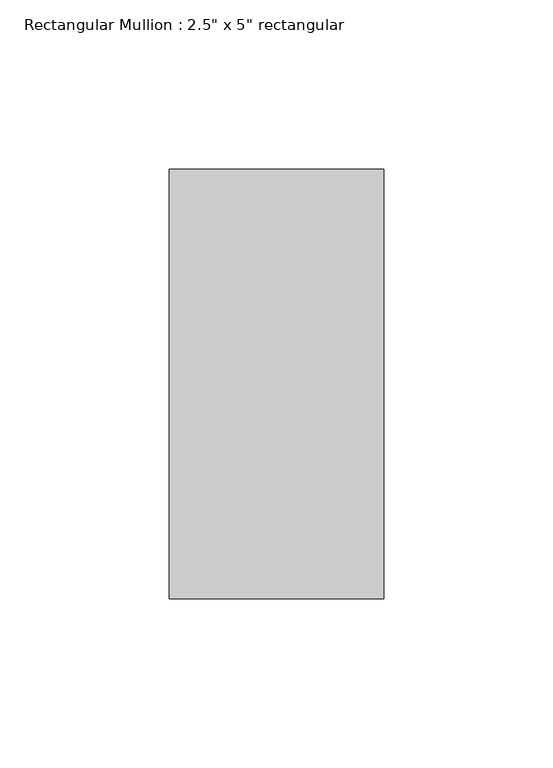
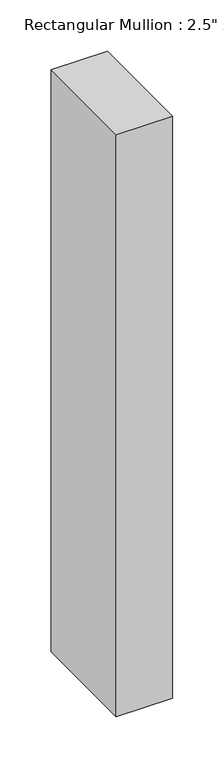
"""IFC4 building model written with IfcOpenShell, lengths in millimetres: member geometry."""

from ifc_helpers import new_model, si_unit, frame, origin, place, context, project, spatial, polyline, outline, extrude, source, transform, mapped, element, save


def member_e97888c9(model_context):
    return source(origin(), model_context, "Body", "SweptSolid", [
        extrude(outline(polyline([(0.0, 63.5), (0.0, -63.5), (-63.5, -63.5), (-63.5, 63.5), (0.0, 63.5)])), frame((0.0, 0.0, -692.4357555), z_axis=(0.0, 0.0, 1.0), x_axis=(1.0, 0.0, 0.0)), (0.0, 0.0, 1.0), 692.4357555),
    ])


if __name__ == "__main__":
    model = new_model("IFC4")
    model_context = context("Model", 3, world=origin())
    ifc_project = project(units=[si_unit("LENGTHUNIT", "METRE", prefix="MILLI")], contexts=[model_context])
    site = spatial("IfcSite", under=ifc_project)
    building = spatial("IfcBuilding", under=site)
    placement = place(None, origin())
    member_shape = member_e97888c9(model_context)
    element("IfcMember", 1, ObjectType="Rectangular Mullion : 2.5\" x 5\" rectangular", at=placement, inside=building, context=model_context, shape_type="MappedRepresentation", body=[
        mapped(member_shape, transform((0.0, 0.0, 0.0), x_axis=(1.0, 0.0, 0.0), y_axis=(0.0, 1.0, 0.0), z_axis=(0.0, 0.0, 1.0))),
    ])
    save(model, "model.ifc")

# Revit data of these elements
# Type "Rectangular Mullion : 2.5\" x 5\" rectangular"
#   built-in parameter 1007304 = 0.416667 (stored number, unit not read)
#   built-in parameter 1007301 = 0.104167 (stored number, unit not read)
#   built-in parameter 1007300 = 0.104167 (stored number, unit not read)
# Element 1 (IfcMember, "Rectangular Mullion : 2.5\" x 5\" rectangular")
#   Materials on its faces: "Aluminum"
# Materials
#   "Aluminum": class "Metal", colour RGB 247 247 247, transparency 0, Description = "Aluminum 6061", Cost = 0
